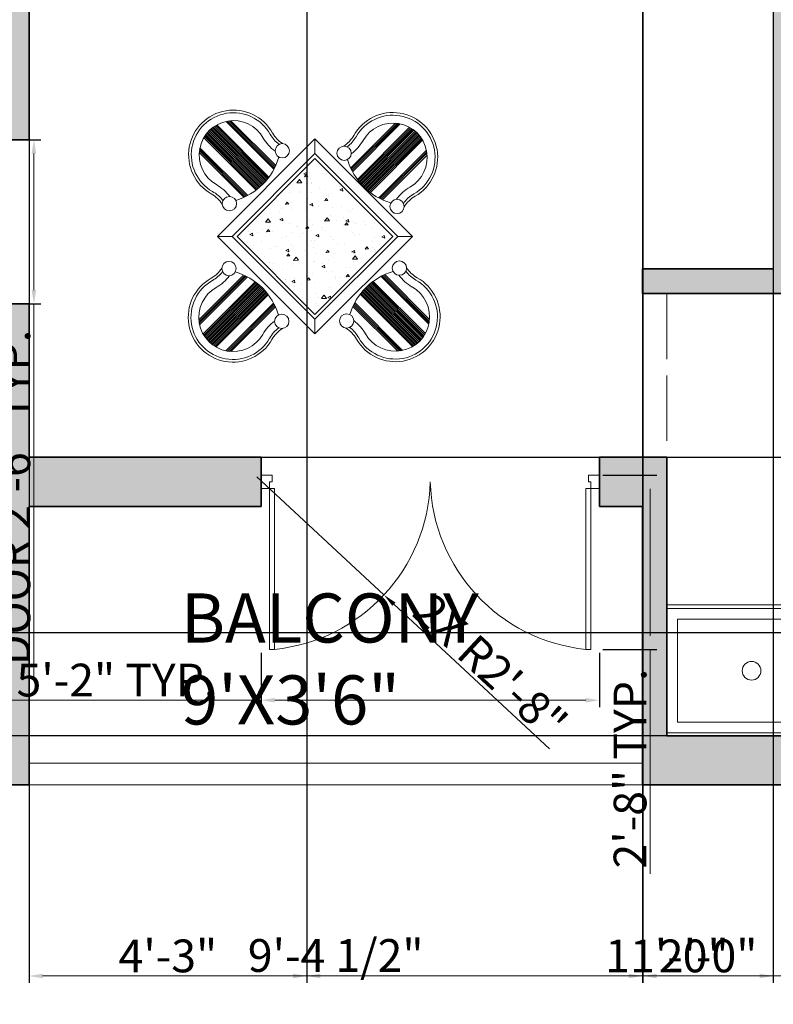
# Model space of a CAD drawing. Units: inches. Extents: x 2696 to 3240, y 1564 to 2310.
# Tile 25 of 76: x 2964 to 3102, y 1565 to 1745. Entities that reach past the tile are written whole.
import ezdxf

# ---------------------------------------------------------------- set-up
doc = ezdxf.new("R2010")
doc.units = ezdxf.units.IN
doc.linetypes.add('ACAD_ISO02W100', pattern=[15, 12, -3])
for name, color, linetype, lineweight in [('A-ANNO-DIMS', 3, 'Continuous', 18), ('A-AREA-IDEN', 7, 'Continuous', 18), ('A-DOOR', 4, 'Continuous', 18), ('A-FLOR-CASE', 8, 'Continuous', 18), ('A-FLOR-FIXT', 8, 'Continuous', 18), ('A-FLOR-HRAL', 7, 'Continuous', 18), ('A-FURN', 251, 'Continuous', 13), ('A-WALL', 7, 'Continuous', 35), ('A-WALL-OVHD', 7, 'ACAD_ISO02W100', 18), ('A-WALL-PATT', 9, 'Continuous', 13)]:
    doc.layers.add(name, color=color, linetype=linetype, lineweight=lineweight)
doc.styles.add('TIMES NEW', font='times.ttf')
doc.styles.add('YQ_DIM', font='SUPEROS.SHX', dxfattribs={"width": 0.8, "bigfont": 'HZDX.SHX'})
doc.dimstyles.new('Siddhuu', dxfattribs={"dimtxt": 6, "dimasz": 2.5, "dimexe": 1.25, "dimexo": 0.625, "dimtad": 1, "dimdec": 1, "dimlunit": 4, "dimtxsty": 'TIMES NEW', "dimcen": 2.5, "dimclrd": 256, "dimclre": 1, "dimclrt": 7, "dimadec": 0, "dimazin": 0, "dimtfac": 1, "dimtdec": 1, "dimtmove": 0, "dimatfit": 3, "dimfxl": 1, "dimtolj": 1, "dimlwd": -1, "dimarcsym": 0})

# ---------------------------------------------------------------- blocks, each defined once
blk = doc.blocks.new('DR_D02')
for p, q in [((-0.46, 0.4948), (-0.475, 0.4948)), ((-0.475, 0.02), (-0.475, 0.4948)), ((-0.46, 0.02), (-0.46, 0.495)), ((0.46, 0.02), (0.46, 0.495)), ((0.46, 0.4948), (0.475, 0.4948)), ((0.475, 0.02), (0.475, 0.4948)), ((-0.46, 0.02), (-0.5, 0.02)), ((-0.5, 0.02), (-0.5, -0.02)), ((-0.475, 0.02), (-0.475, 0)), ((-0.475, 0), (-0.4675, 0)), ((-0.4675, 0), (-0.4675, -0.02)), ((0.46, 0.02), (0.5, 0.02)), ((0.4675, 0), (0.4675, -0.02)), ((0.475, 0), (0.4675, 0)), ((0.475, 0.02), (0.475, 0)), ((0.5, 0.02), (0.5, -0.02)), ((-0.4675, -0.02), (-0.5, -0.02)), ((0.4675, -0.02), (0.5, -0.02))]:
    blk.add_line(p, q)
for centre, start, end in [((-0.5121, -0.0149), 1.6619, 84.1677), ((0.5121, -0.0149), 95.8323, 178.3381)]:
    blk.add_arc(centre, 0.5123, start, end)
blk = doc.blocks.new('DINING-SET-4')
h = blk.add_hatch()
h.set_pattern_fill('AR-CONC,_O', color=256, scale=0.03156, angle=135)
h.set_pattern_definition([(185, (694.1166, -47.9622), (-3.709933, 4.421326), [0.60121, -6.613307]), (130, (694.1166, -47.962), (-3.47714, -5.050095), [0.48097, -5.290645]), (235.451, (693.8074, -47.594), (-7.187067, -0.628735), [0.51095, -5.620443]), (181.1842, (692.983, -49.096), (-5.11118, 6.98761), [0.90181, -9.91996]), (231.6356, (692.557, -48.514), (-10.81945, -0.22364), [0.76642, -8.43066]), (126.184, (692.983, -49.096), (-10.81945, -0.22362), [0.72145, -7.93597]), (156, (692.6995, -48.2457), (-1.10128, 5.66559), [0.60121, -6.613307]), (101, (692.6995, -48.2457), (-5.48951, -2.73116), [0.48097, -5.290645]), (206.4514, (692.608, -47.7735), (-6.590787, 2.93441), [0.51095, -5.620443]), (172.5, (694.1166, -47.9622), (-1.955854, -1.8180035), [0, -5.226516, 0, -5.370807, 0, -5.310686]), (142.5, (694.1166, -47.9622), (-3.726774, -0.744482), [0, -3.062161, 0, -5.106274, 0, -2.024073]), (102.5, (695.3806, -49.2263), (-2.8979947, 3.15368), [0, -2.004032, 0, -6.25258, 0, -8.296694]), (92.5, (695.9475, -49.793), (-3.873065, 2.73823), [0, -2.605242, 0, -4.152355, 0, -5.891855])])
h.paths.add_polyline_path([(23.22, 8.74), (37.5, 23.02), (23.22, 37.31), (8.94, 23.02)])
for p, q in [((14.65, 33.71), (5.03, 43.33)), ((14.79, 33.91), (5.25, 43.45)), ((15.69, 35.33), (6.93, 44.09)), ((15.81, 35.56), (7.22, 44.15)), ((15.92, 35.79), (7.52, 44.19)), ((16.03, 36.02), (7.83, 44.22)), ((29.77, 35.57), (37.97, 43.77)), ((29.88, 35.34), (38.28, 43.74)), ((29.99, 35.11), (38.58, 43.7)), ((30.11, 34.88), (38.86, 43.64)), ((12.8, 31.8), (3.1, 41.5)), ((12.99, 31.96), (3.24, 41.7)), ((13.17, 32.12), (3.39, 41.89)), ((13.35, 32.28), (3.55, 42.08)), ((13.52, 32.45), (3.71, 42.26)), ((13.69, 32.62), (3.88, 42.43)), ((13.86, 32.79), (4.05, 42.6)), ((14.03, 32.97), (4.24, 42.76)), ((14.19, 33.15), (4.42, 42.91)), ((14.34, 33.33), (4.62, 43.06)), ((14.5, 33.52), (4.82, 43.2)), ((31, 33.46), (40.55, 43.01)), ((31.15, 33.26), (40.76, 42.88)), ((31.3, 33.07), (40.97, 42.75)), ((31.45, 32.88), (41.18, 42.61)), ((31.61, 32.7), (41.37, 42.46)), ((31.77, 32.52), (41.56, 42.31)), ((31.93, 32.34), (41.74, 42.15)), ((32.1, 32.17), (41.92, 41.98)), ((32.27, 32), (42.09, 41.81)), ((32.45, 31.83), (42.25, 41.63)), ((12.42, 31.5), (2.84, 41.08)), ((12.61, 31.65), (2.97, 41.3)), ((23.22, 38.2), (23.22, 40.88)), ((32.63, 31.67), (42.4, 41.45)), ((32.81, 31.51), (42.55, 41.25)), ((32.99, 31.35), (42.69, 41.05)), ((33.18, 31.2), (42.83, 40.85)), ((33.38, 31.05), (42.96, 40.63)), ((10.21, 30.19), (2.02, 38.38)), ((10.44, 30.3), (2.05, 38.7)), ((10.67, 30.41), (2.09, 39)), ((10.9, 30.53), (2.15, 39.28)), ((34.9, 30.08), (43.65, 38.83)), ((35.12, 29.96), (43.7, 38.55)), ((35.35, 29.85), (43.75, 38.25)), ((35.58, 29.74), (43.78, 37.94)), ((8.05, 23.02), (5.37, 23.02)), ((38.4, 23.02), (41.07, 23.02)), ((10.15, 15.95), (1.95, 7.75)), ((10.38, 15.84), (1.98, 7.44)), ((10.61, 15.73), (2.02, 7.14)), ((10.84, 15.61), (2.08, 6.86)), ((12.26, 14.72), (2.71, 5.17)), ((12.46, 14.57), (2.84, 4.95)), ((33.51, 14.5), (43.19, 4.83)), ((33.7, 14.65), (43.32, 5.04)), ((33.9, 14.8), (43.45, 5.25)), ((35.33, 15.7), (44.08, 6.94)), ((35.55, 15.81), (44.14, 7.23)), ((35.78, 15.93), (44.18, 7.52)), ((36.01, 16.03), (44.21, 7.83)), ((12.65, 14.42), (2.97, 4.75)), ((12.83, 14.27), (3.11, 4.54)), ((13.02, 14.11), (3.26, 4.35)), ((13.2, 13.95), (3.41, 4.16)), ((13.38, 13.78), (3.57, 3.98)), ((13.55, 13.62), (3.74, 3.8)), ((13.72, 13.45), (3.91, 3.63)), ((13.89, 13.27), (4.09, 3.47)), ((14.05, 13.09), (4.27, 3.32)), ((14.21, 12.91), (4.47, 3.17)), ((14.36, 12.72), (4.67, 3.03)), ((31.8, 12.81), (41.5, 3.11)), ((31.95, 12.99), (41.69, 3.25)), ((32.11, 13.18), (41.89, 3.4)), ((32.27, 13.35), (42.07, 3.55)), ((32.44, 13.53), (42.25, 3.72)), ((32.61, 13.7), (42.42, 3.89)), ((32.78, 13.87), (42.59, 4.06)), ((32.96, 14.03), (42.75, 4.24)), ((33.14, 14.19), (42.9, 4.43)), ((33.33, 14.35), (43.05, 4.63)), ((14.52, 12.54), (4.87, 2.89)), ((14.67, 12.34), (5.08, 2.76)), ((15.64, 10.82), (6.89, 2.07)), ((30.52, 10.91), (39.27, 2.15)), ((31.49, 12.43), (41.08, 2.85)), ((31.64, 12.62), (41.29, 2.97)), ((15.75, 10.6), (7.17, 2.02)), ((15.87, 10.37), (7.47, 1.97)), ((15.98, 10.14), (7.78, 1.94)), ((30.18, 10.22), (38.38, 2.03)), ((30.29, 10.45), (38.69, 2.06)), ((30.41, 10.68), (38.99, 2.1)), ((23.22, 7.85), (23.22, 5.17))]:
    blk.add_line(p, q)
for points in [[(41.07, 23.02), (23.22, 40.88), (5.37, 23.02), (23.22, 5.17)], [(38.4, 23.02), (23.22, 38.2), (8.05, 23.02), (23.22, 7.85)], [(37.5, 23.02), (23.22, 37.31), (8.94, 23.02), (23.22, 8.74)]]:
    blk.add_lwpolyline(points, close=True)
for centre in [(17.23, 38.71), (28.57, 38.26), (7.55, 29.03), (38.27, 28.51), (7.46, 17.15), (38.7, 17.23), (17.14, 7.47), (29.03, 7.55)]:
    blk.add_circle(centre, 1.31)
for centre, radius, start, end in [((8.28, 37.96), 8.21, 29.1881, 240.1532), ((8.28, 37.96), 7.72, 29.1881, 240.1532), ((37.51, 37.51), 8.21, 299.8468, 150.8119), ((37.51, 37.51), 7.72, 299.8468, 150.8119), ((8.28, 37.96), 6.28, 29.2752, 240.1505), ((37.51, 37.51), 6.28, 299.8495, 150.7248), ((20.45, 44.88), 6.28, 210.1015, 232.6572), ((20.45, 44.88), 5.79, 210.1015, 236.9513), ((25.34, 44.43), 5.79, 303.0487, 329.8985), ((20.45, 44.88), 7.72, 209.8594, 234.0675), ((25.34, 44.43), 6.28, 307.3428, 329.8985), ((25.34, 44.43), 7.72, 305.9325, 330.1406), ((5.4, 40.81), 11.66, 286.5158, 343.8317), ((40.4, 40.36), 11.66, 196.1683, 253.4842), ((1.37, 25.79), 7.72, 36.1055, 60.6071), ((1.37, 25.79), 5.79, 32.6748, 60.7093), ((1.37, 25.79), 6.28, 37.2611, 60.7093), ((44.43, 25.34), 7.72, 119.3929, 143.8945), ((44.43, 25.34), 6.28, 119.2907, 142.7389), ((44.43, 25.34), 5.79, 119.2907, 147.3252), ((1.29, 20.38), 5.79, 300.1015, 326.9513), ((1.29, 20.38), 6.28, 300.1015, 322.6572), ((5.36, 5.32), 11.66, 16.5158, 73.8317), ((40.8, 5.4), 11.66, 106.1683, 163.4842), ((44.87, 20.46), 6.28, 217.3428, 239.8985), ((44.87, 20.46), 5.79, 213.0487, 239.8985), ((8.21, 8.21), 8.21, 119.1881, 330.1532), ((8.21, 8.21), 7.72, 119.1881, 330.1532), ((1.29, 20.38), 7.72, 299.8594, 324.0675), ((37.95, 8.29), 8.21, 209.8468, 60.8119), ((37.95, 8.29), 7.72, 209.8468, 60.8119), ((44.87, 20.46), 7.72, 215.9325, 240.1406), ((8.21, 8.21), 6.28, 119.2752, 330.1505), ((37.95, 8.29), 6.28, 209.8495, 60.7248), ((20.38, 1.29), 7.72, 126.1055, 150.6071), ((25.78, 1.37), 7.72, 29.3929, 53.8945), ((20.38, 1.29), 6.28, 127.2611, 150.7093), ((20.38, 1.29), 5.79, 122.6748, 150.7093), ((25.78, 1.37), 5.79, 29.2907, 57.3252), ((25.78, 1.37), 6.28, 29.2907, 52.7389)]:
    blk.add_arc(centre, radius, start, end)
blk = doc.blocks.new('SINK-KITCHEN')
for points in [[(0, 22.8), (31.04, 22.8), (31.04, 0), (0, 0)], [(1.97, 20.82), (29.07, 20.82), (29.07, 1.97), (1.97, 1.97)]]:
    blk.add_lwpolyline(points, close=True)
blk.add_circle((15.52, 11.4), 1.71)
blk = doc.blocks.new('*D32')
at = {"layer": 'A-ANNO-DIMS', "color": 1, "lineweight": -2, "transparency": 16777216}
for p, q in [((2962.73, 1723.33), (2967.86, 1723.33)), ((2962.73, 1693.33), (2967.86, 1693.33))]:
    blk.add_line(p, q, dxfattribs=at)
at = {"layer": 'A-ANNO-DIMS', "transparency": 16777216}
for p, q in [((2966.61, 1720.83), (2966.61, 1695.83)), ((2966.61, 1693.33), (2966.61, 1624.85))]:
    blk.add_line(p, q, dxfattribs=at)
for points in [[(2966.19, 1720.83), (2967.03, 1720.83), (2966.61, 1723.33)], [(2966.19, 1695.83), (2967.03, 1695.83), (2966.61, 1693.33)]]:
    blk.add_solid(points, dxfattribs=at)
at = {"layer": 'Defpoints', "color": 0, "transparency": 16777216}
for p in [(2962.11, 1723.33), (2962.11, 1693.33), (2966.61, 1693.33)]:
    blk.add_point(p, dxfattribs=at)
at = {"layer": 'A-ANNO-DIMS', "color": 7, "transparency": 16777216, "insert": (2962.92, 1657.84), "char_height": 6, "attachment_point": 5, "rotation": 90, "style": 'TIMES NEW'}
blk.add_mtext('\\A1;DOOR 2\'-6" TYP.', dxfattribs=at)
blk = doc.blocks.new('*D36')
at = {"layer": 'A-ANNO-DIMS', "color": 1, "lineweight": -2, "transparency": 16777216}
for p, q in [((3008.24, 1629.39), (3008.24, 1619.46)), ((3070.24, 1629.39), (3070.24, 1619.46))]:
    blk.add_line(p, q, dxfattribs=at)
at = {"layer": 'A-ANNO-DIMS', "transparency": 16777216}
for p, q in [((3008.24, 1620.71), (2894.72, 1620.71)), ((3067.74, 1620.71), (3010.74, 1620.71))]:
    blk.add_line(p, q, dxfattribs=at)
for points in [[(3010.74, 1621.13), (3010.74, 1620.29), (3008.24, 1620.71)], [(3067.74, 1621.13), (3067.74, 1620.29), (3070.24, 1620.71)]]:
    blk.add_solid(points, dxfattribs=at)
at = {"layer": 'Defpoints', "color": 0, "transparency": 16777216}
for p in [(3008.24, 1630.01), (3070.24, 1630.01), (3008.24, 1620.71)]:
    blk.add_point(p, dxfattribs=at)
at = {"layer": 'A-ANNO-DIMS', "color": 7, "transparency": 16777216, "insert": (2950.23, 1624.4), "char_height": 6, "attachment_point": 5, "style": 'TIMES NEW'}
blk.add_mtext('\\A1;BALCONY DOOR 5\'-2" TYP.', dxfattribs=at)
blk = doc.blocks.new('*D37')
at = {"layer": 'A-ANNO-DIMS', "color": 1, "lineweight": -2, "transparency": 16777216}
for p, q in [((3070.86, 1661.94), (3080.79, 1661.94)), ((3070.86, 1630.01), (3080.79, 1630.01))]:
    blk.add_line(p, q, dxfattribs=at)
at = {"layer": 'A-ANNO-DIMS', "transparency": 16777216}
for p, q in [((3079.54, 1659.44), (3079.54, 1632.51)), ((3079.54, 1630.01), (3079.54, 1588.89))]:
    blk.add_line(p, q, dxfattribs=at)
for points in [[(3079.12, 1659.44), (3079.95, 1659.44), (3079.54, 1661.94)], [(3079.12, 1632.51), (3079.95, 1632.51), (3079.54, 1630.01)]]:
    blk.add_solid(points, dxfattribs=at)
at = {"layer": 'Defpoints', "color": 0, "transparency": 16777216}
for p in [(3070.24, 1661.94), (3070.24, 1630.01), (3079.54, 1630.01)]:
    blk.add_point(p, dxfattribs=at)
at = {"layer": 'A-ANNO-DIMS', "color": 7, "transparency": 16777216, "insert": (3075.85, 1608.2), "char_height": 6, "attachment_point": 5, "rotation": 90, "style": 'TIMES NEW'}
blk.add_mtext('\\A1;2\'-8" TYP.', dxfattribs=at)
blk = doc.blocks.new('*D50')
at = {"layer": 'A-ANNO-DIMS', "color": 1, "lineweight": -2, "transparency": 16777216}
for p, q in [((2965.71, 1979.58), (2965.71, 1568.95)), ((3016.61, 1979.58), (3016.61, 1568.95))]:
    blk.add_line(p, q, dxfattribs=at)
at = {"layer": 'A-ANNO-DIMS', "transparency": 16777216}
blk.add_line((2968.21, 1570.2), (3014.11, 1570.2), dxfattribs=at)
for points in [[(2968.21, 1570.62), (2968.21, 1569.78), (2965.71, 1570.2)], [(3014.11, 1570.62), (3014.11, 1569.78), (3016.61, 1570.2)]]:
    blk.add_solid(points, dxfattribs=at)
at = {"layer": 'Defpoints', "color": 0, "transparency": 16777216}
for p in [(2965.71, 1980.2), (3016.61, 1980.2), (3016.61, 1570.2)]:
    blk.add_point(p, dxfattribs=at)
at = {"layer": 'A-ANNO-DIMS', "color": 7, "transparency": 16777216, "insert": (2991.16, 1573.88), "char_height": 6, "attachment_point": 5, "style": 'TIMES NEW'}
blk.add_mtext('\\A1;4\'-3"', dxfattribs=at)
blk = doc.blocks.new('*D51')
at = {"layer": 'A-ANNO-DIMS', "color": 1, "lineweight": -2, "transparency": 16777216}
for p, q in [((3016.61, 1979.58), (3016.61, 1568.95)), ((3148.61, 1979.58), (3148.61, 1568.95))]:
    blk.add_line(p, q, dxfattribs=at)
at = {"layer": 'A-ANNO-DIMS', "transparency": 16777216}
blk.add_line((3019.11, 1570.2), (3146.11, 1570.2), dxfattribs=at)
for points in [[(3019.11, 1570.62), (3019.11, 1569.78), (3016.61, 1570.2)], [(3146.11, 1570.62), (3146.11, 1569.78), (3148.61, 1570.2)]]:
    blk.add_solid(points, dxfattribs=at)
at = {"layer": 'Defpoints', "color": 0, "transparency": 16777216}
for p in [(3016.61, 1980.2), (3148.61, 1980.2), (3148.61, 1570.2)]:
    blk.add_point(p, dxfattribs=at)
at = {"layer": 'A-ANNO-DIMS', "color": 7, "transparency": 16777216, "insert": (3082.61, 1573.88), "char_height": 6, "attachment_point": 5, "style": 'TIMES NEW'}
blk.add_mtext('\\A1;11\'-0"', dxfattribs=at)
blk = doc.blocks.new('*D56')
at = {"layer": 'A-ANNO-DIMS', "color": 1, "lineweight": -2, "transparency": 16777216}
for p, q in [((2966.33, 1884.2), (3235.86, 1884.2)), ((2966.33, 1665.2), (3235.86, 1665.2))]:
    blk.add_line(p, q, dxfattribs=at)
at = {"layer": 'A-ANNO-DIMS', "transparency": 16777216}
blk.add_line((3234.61, 1667.7), (3234.61, 1881.7), dxfattribs=at)
for points in [[(3234.19, 1881.7), (3235.03, 1881.7), (3234.61, 1884.2)], [(3234.19, 1667.7), (3235.03, 1667.7), (3234.61, 1665.2)]]:
    blk.add_solid(points, dxfattribs=at)
at = {"layer": 'Defpoints', "color": 0, "transparency": 16777216}
for p in [(2965.71, 1884.2), (3234.61, 1884.2), (2965.71, 1665.2)]:
    blk.add_point(p, dxfattribs=at)
at = {"layer": 'A-ANNO-DIMS', "color": 7, "transparency": 16777216, "insert": (3230.93, 1774.7), "char_height": 6, "attachment_point": 5, "rotation": 90, "style": 'TIMES NEW'}
blk.add_mtext('\\A1;18\'-3"', dxfattribs=at)
blk = doc.blocks.new('*D65')
at = {"layer": 'A-ANNO-DIMS', "color": 1, "lineweight": -2, "transparency": 16777216}
for p, q in [((3078.21, 2122.08), (3078.21, 1568.95)), ((3102.11, 2122.08), (3102.11, 1568.95))]:
    blk.add_line(p, q, dxfattribs=at)
at = {"layer": 'A-ANNO-DIMS', "transparency": 16777216}
blk.add_line((3080.71, 1570.2), (3099.61, 1570.2), dxfattribs=at)
for points in [[(3080.71, 1570.62), (3080.71, 1569.78), (3078.21, 1570.2)], [(3099.61, 1570.62), (3099.61, 1569.78), (3102.11, 1570.2)]]:
    blk.add_solid(points, dxfattribs=at)
at = {"layer": 'Defpoints', "color": 0, "transparency": 16777216}
for p in [(3078.21, 2122.7), (3102.11, 2122.7), (3102.11, 1570.2)]:
    blk.add_point(p, dxfattribs=at)
at = {"layer": 'A-ANNO-DIMS', "color": 7, "transparency": 16777216, "insert": (3090.16, 1573.88), "char_height": 6, "attachment_point": 5, "style": 'TIMES NEW'}
blk.add_mtext('\\A1;2\'-0"', dxfattribs=at)
blk = doc.blocks.new('*D67')
at = {"layer": 'A-ANNO-DIMS', "color": 1, "lineweight": -2, "transparency": 16777216}
for p, q in [((2965.71, 1883.58), (2965.71, 1568.95)), ((3078.11, 1791.45), (3078.11, 1568.95))]:
    blk.add_line(p, q, dxfattribs=at)
at = {"layer": 'A-ANNO-DIMS', "transparency": 16777216}
blk.add_line((2968.21, 1570.2), (3075.61, 1570.2), dxfattribs=at)
for points in [[(2968.21, 1570.62), (2968.21, 1569.78), (2965.71, 1570.2)], [(3075.61, 1570.62), (3075.61, 1569.78), (3078.11, 1570.2)]]:
    blk.add_solid(points, dxfattribs=at)
at = {"layer": 'Defpoints', "color": 0, "transparency": 16777216}
for p in [(2965.71, 1884.2), (3078.11, 1792.08), (3078.11, 1570.2)]:
    blk.add_point(p, dxfattribs=at)
at = {"layer": 'A-ANNO-DIMS', "color": 7, "transparency": 16777216, "insert": (3021.91, 1573.96), "char_height": 6, "attachment_point": 5, "style": 'TIMES NEW'}
blk.add_mtext('\\A1;9\'-4 1/2"', dxfattribs=at)
blk = doc.blocks.new('*D81')
at = {"layer": 'A-ANNO-DIMS', "color": 1, "lineweight": -2, "transparency": 16777216}
for p, q in [((3189.99, 1633.05), (2709.36, 1633.05)), ((3189.99, 1614.2), (2709.36, 1614.2))]:
    blk.add_line(p, q, dxfattribs=at)
at = {"layer": 'A-ANNO-DIMS', "transparency": 16777216}
blk.add_line((2710.61, 1616.7), (2710.61, 1630.55), dxfattribs=at)
for points in [[(2710.19, 1630.55), (2711.03, 1630.55), (2710.61, 1633.05)], [(2710.19, 1616.7), (2711.03, 1616.7), (2710.61, 1614.2)]]:
    blk.add_solid(points, dxfattribs=at)
at = {"layer": 'Defpoints', "color": 0, "transparency": 16777216}
for p in [(2710.61, 1633.05), (3190.61, 1633.05), (3190.61, 1614.2)]:
    blk.add_point(p, dxfattribs=at)
at = {"layer": 'A-ANNO-DIMS', "color": 7, "transparency": 16777216, "insert": (2706.93, 1623.62), "char_height": 6, "attachment_point": 5, "rotation": 90, "style": 'TIMES NEW'}
blk.add_mtext('\\A1;1\'-7"', dxfattribs=at)
blk = doc.blocks.new('*D84')
at = {"layer": 'A-ANNO-DIMS', "transparency": 16777216}
for p, q in [((3007.49, 1661.62), (3030.75, 1640)), ((3061.1, 1611.78), (3032.58, 1638.29))]:
    blk.add_line(p, q, dxfattribs=at)
blk.add_solid([(3032.87, 1638.6), (3032.3, 1637.99), (3030.75, 1640)], dxfattribs=at)
at = {"layer": 'Defpoints', "color": 0, "transparency": 16777216}
for p in [(3007.49, 1661.62), (3030.75, 1640)]:
    blk.add_point(p, dxfattribs=at)
at = {"layer": 'A-ANNO-DIMS', "color": 7, "transparency": 16777216, "insert": (3050.26, 1626.88), "char_height": 6, "attachment_point": 5, "rotation": 317.0859, "style": 'TIMES NEW'}
blk.add_mtext('\\A1;2X R2\'-8"', dxfattribs=at)

msp = doc.modelspace()

# ---------------------------------------------------------------- hatches: boundary and pattern name
at = {"layer": 'A-WALL-PATT', "transparency": 33554556}
h = msp.add_hatch(color=256, dxfattribs=at)
h.dxf.hatch_style = 1
h.paths.add_polyline_path([(2879.11, 2253.2), (2905.91, 2253.2), (2905.91, 2262.2), (2841.89, 2262.2), (2841.89, 2253.2), (2870.11, 2253.2), (2870.11, 2176.6), (2965.71, 2176.6), (2965.71, 2206.7), (2973.58, 2206.7), (2973.58, 2215.7), (2965.71, 2215.7), (2965.71, 2262.2), (2929.91, 2262.2), (2929.91, 2253.2), (2956.71, 2253.2), (2956.71, 2185.6), (2879.11, 2185.6)])
h.paths.add_polyline_path([(2782.83, 2262.2), (2745.61, 2262.2), (2745.61, 2228.73), (2754.61, 2228.73), (2754.61, 2253.2), (2782.83, 2253.2)])
h.paths.add_polyline_path([(2754.61, 2136.2), (2965.71, 2136.2), (2965.71, 2145.2), (2879.11, 2145.2), (2879.11, 2147.07), (2877.34, 2147.07), (2870.11, 2147.07), (2870.11, 2145.2), (2754.61, 2145.2), (2754.61, 2169.67), (2745.61, 2169.67), (2745.61, 2000.2), (2754.61, 2000.2), (2754.61, 2019.2), (2849.08, 2019.2), (2849.08, 2023.7), (2841.21, 2023.7), (2841.21, 2051.83), (2836.71, 2051.83), (2836.71, 2023.7), (2754.61, 2023.7), (2754.61, 2091.2), (2836.71, 2091.2), (2836.71, 2087.83), (2841.21, 2087.83), (2841.21, 2095.7), (2754.61, 2095.7)])
h.paths.add_polyline_path([(2965.71, 2136.2), (2956.71, 2136.2), (2956.71, 2023.7), (2885.08, 2023.7), (2885.08, 2019.2), (2956.71, 2019.2), (2956.71, 1950.58), (2965.71, 1950.58), (2965.71, 1980.2), (2973.58, 1980.2), (2973.58, 1989.2), (2965.71, 1989.2)])
h.paths.add_polyline_path([(2754.61, 1906.7), (2880.21, 1906.7), (2884.71, 1906.7), (2956.71, 1906.7), (2956.71, 1792.7), (2944.71, 1792.7), (2944.71, 1783.7), (2956.71, 1783.7), (2956.71, 1740.2), (2884.71, 1740.2), (2884.71, 1783.7), (2896.71, 1783.7), (2896.71, 1792.7), (2884.71, 1792.7), (2884.71, 1846.7), (2880.21, 1846.7), (2880.21, 1740.2), (2754.61, 1740.2), (2754.61, 1777.2), (2745.61, 1777.2), (2745.61, 1692.7), (2754.61, 1692.7), (2754.61, 1731.2), (2956.71, 1731.2), (2956.71, 1723.33), (2965.71, 1723.33), (2965.71, 1884.2), (2973.58, 1884.2), (2973.58, 1893.2), (2965.71, 1893.2), (2965.71, 1914.58), (2956.71, 1914.58), (2956.71, 1911.2), (2754.61, 1911.2), (2754.61, 1930.2), (2745.61, 1930.2), (2745.61, 1817.2), (2754.61, 1817.2), (2754.61, 1854.2), (2826.61, 1854.2), (2826.61, 1868.83), (2822.11, 1868.83), (2822.11, 1858.7), (2754.61, 1858.7)])
h.paths.add_polyline_path([(2965.71, 1656.2), (3008.24, 1656.2), (3008.24, 1665.2), (2965.71, 1665.2), (2965.71, 1693.33), (2956.71, 1693.33), (2956.71, 1686.2), (2934.58, 1686.2), (2934.58, 1681.7), (2956.71, 1681.7), (2956.71, 1614.2), (2896.71, 1614.2), (2896.71, 1681.7), (2904.58, 1681.7), (2904.58, 1686.2), (2892.21, 1686.2), (2892.21, 1614.2), (2858.41, 1614.2), (2858.41, 1605.2), (2965.71, 1605.2)])
h.paths.add_polyline_path([(2788.41, 1614.2), (2754.61, 1614.2), (2754.61, 1652.7), (2745.61, 1652.7), (2745.61, 1605.2), (2788.41, 1605.2)])
h.paths.add_polyline_path([(3199.61, 1633.05), (3190.61, 1633.05), (3190.61, 1614.2), (3082.61, 1614.2), (3082.61, 1665.2), (3070.24, 1665.2), (3070.24, 1656.2), (3078.11, 1656.2), (3078.11, 1605.2), (3199.61, 1605.2)])
h.paths.add_polyline_path([(3199.61, 1702.05), (3190.61, 1702.05), (3190.61, 1699.7), (3106.61, 1699.7), (3106.61, 1747.7), (3190.61, 1747.7), (3190.61, 1752.2), (3082.61, 1752.2), (3082.61, 1760.08), (3078.11, 1760.08), (3078.11, 1747.7), (3102.11, 1747.7), (3102.11, 1699.7), (3078.11, 1699.7), (3078.11, 1695.2), (3190.61, 1695.2), (3190.61, 1676.35), (3199.61, 1676.35)])
h.paths.add_polyline_path([(3199.61, 1783.2), (3190.61, 1783.2), (3190.61, 1745.35), (3199.61, 1745.35)])
h.paths.add_polyline_path([(3082.61, 1884.2), (3190.61, 1884.2), (3190.61, 1853.2), (3199.61, 1853.2), (3199.61, 1901.7), (3190.61, 1901.7), (3190.61, 1893.2), (3005.58, 1893.2), (3005.58, 1891.28), (3005.58, 1884.2), (3078.11, 1884.2), (3078.11, 1792.08), (3082.61, 1792.08)])
h.paths.add_polyline_path([(3199.61, 1994.7), (3190.61, 1994.7), (3190.61, 1989.2), (3073.71, 1989.2), (3073.71, 2034.2), (3069.21, 2034.2), (3069.21, 1989.2), (3005.58, 1989.2), (3005.58, 1980.2), (3190.61, 1980.2), (3190.61, 1971.7), (3199.61, 1971.7)])
h.paths.add_polyline_path([(3199.61, 2155.2), (3190.61, 2155.2), (3190.61, 2064.7), (3199.61, 2064.7)])
h.paths.add_polyline_path([(3190.61, 2074.7), (3106.61, 2074.7), (3106.61, 2122.7), (3190.61, 2122.7), (3190.61, 2127.2), (3082.71, 2127.2), (3082.71, 2135.08), (3073.71, 2135.08), (3073.71, 2122.7), (3102.11, 2122.7), (3102.11, 2074.7), (3069.21, 2074.7), (3069.21, 2070.2), (3190.61, 2070.2)])
h.paths.add_polyline_path([(3082.71, 2253.2), (3190.61, 2253.2), (3190.61, 2225.2), (3199.61, 2225.2), (3199.61, 2262.2), (3073.71, 2262.2), (3073.71, 2215.7), (3035.58, 2215.7), (3035.58, 2206.7), (3073.71, 2206.7), (3073.71, 2171.08), (3082.71, 2171.08)])

# ---------------------------------------------------------------- linework, layer by layer
at = {"layer": 'A-FLOR-CASE'}
msp.add_line((3082.61, 1638.2), (3166.61, 1638.2), dxfattribs=at)
at = {"layer": 'A-FLOR-HRAL'}
for p, q in [((2965.71, 1609.2), (3078.11, 1609.2)), ((2965.71, 1605.2), (3078.11, 1605.2))]:
    msp.add_line(p, q, dxfattribs=at)
at = {"layer": 'A-WALL'}
for p, q in [((2965.71, 1884.2), (2965.71, 1723.33)), ((2956.71, 1723.33), (2965.71, 1723.33)), ((3078.11, 1699.7), (3102.11, 1699.7)), ((3078.11, 1695.2), (3078.11, 1699.7)), ((3078.11, 1695.2), (3190.61, 1695.2)), ((2956.71, 1693.33), (2965.71, 1693.33)), ((2965.71, 1693.33), (2965.71, 1665.2)), ((2965.71, 1665.2), (3008.24, 1665.2)), ((3008.24, 1665.2), (3008.24, 1656.2)), ((3070.24, 1665.2), (3082.61, 1665.2)), ((3070.24, 1665.2), (3070.24, 1656.2)), ((3082.61, 1614.2), (3082.61, 1665.2)), ((2965.71, 1656.2), (3008.24, 1656.2)), ((2965.71, 1656.2), (2965.71, 1605.2)), ((3070.24, 1656.2), (3078.11, 1656.2)), ((3078.11, 1605.2), (3078.11, 1656.2)), ((3082.61, 1614.2), (3190.61, 1614.2)), ((2858.41, 1605.2), (2965.71, 1605.2)), ((3078.11, 1605.2), (3199.61, 1605.2))]:
    msp.add_line(p, q, dxfattribs=at)
at = {"layer": 'A-WALL-OVHD'}
for p, q in [((3078.11, 1695.2), (3078.11, 1665.2)), ((3082.61, 1695.2), (3082.61, 1665.2))]:
    msp.add_line(p, q, dxfattribs=at)

# ---------------------------------------------------------------- block references
at = {"layer": 'A-DOOR', "xscale": 62, "yscale": 62, "zscale": 62, "rotation": 180.0000000000002}
msp.add_blockref('DR_D02', (3039.24, 1660.7), dxfattribs=at)
at = {"layer": 'A-FLOR-FIXT'}
msp.add_blockref('SINK-KITCHEN', (3082.61, 1614.71), dxfattribs=at)
at = {"layer": 'A-FURN'}
msp.add_blockref('DINING-SET-4', (2994.89, 1682.63), dxfattribs=at)

# ---------------------------------------------------------------- texts
at = {"layer": 'A-AREA-IDEN', "insert": (2993.57, 1640.27), "char_height": 9, "attachment_point": 1, "style": 'YQ_DIM'}
msp.add_mtext_dynamic_manual_height_columns('BALCONY\\P9\'X3\'6"', width=48.0032, gutter_width=12.5, heights=[0], dxfattribs=at)

# ---------------------------------------------------------------- dimensions: what is measured, and where the dimension line sits
at = {"layer": 'A-ANNO-DIMS'}
for base, p1, p2, picture, middle in [((3102.11, 1570.2), (3078.21, 2122.7), (3102.11, 2122.7), '*D65', (3090.16, 1573.88)), ((3016.61, 1570.2), (2965.71, 1980.2), (3016.61, 1980.2), '*D50', (2991.16, 1573.88)), ((3148.61, 1570.2), (3016.61, 1980.2), (3148.61, 1980.2), '*D51', (3082.61, 1573.88)), ((3078.11, 1570.2), (2965.71, 1884.2), (3078.11, 1792.08), '*D67', (3021.91, 1573.96))]:
    dim = msp.add_linear_dim(base=base, p1=p1, p2=p2, dimstyle='Siddhuu', override={"dimdec": 1, "dimlfac": 1, "dimrnd": 0, "dimzin": 1, "dimdsep": 46, "dimlunit": 4, "dimfrac": 2}, dxfattribs=at)
    dim.commit()
    dim.dimension.update_dxf_attribs({"geometry": picture, "text_midpoint": middle})
for base, p1, p2, picture, middle in [((3234.61, 1884.2), (2965.71, 1665.2), (2965.71, 1884.2), '*D56', (3230.93, 1774.7)), ((2710.6114, 1633.0476), (3190.6114, 1614.2011), (3190.6114, 1633.0476), '*D81', (2706.9258, 1623.6243))]:
    dim = msp.add_linear_dim(base=base, p1=p1, p2=p2, angle=90, dimstyle='Siddhuu', override={"dimdec": 1, "dimlfac": 1, "dimrnd": 0, "dimzin": 1, "dimdsep": 46, "dimlunit": 4, "dimfrac": 2}, dxfattribs=at)
    dim.commit()
    dim.dimension.update_dxf_attribs({"geometry": picture, "text_midpoint": middle})
for base, p1, p2, angle, text, picture, middle in [((2966.61, 1693.33), (2962.11, 1723.33), (2962.11, 1693.33), 270, 'DOOR <> TYP.', '*D32', (2962.92, 1657.84)), ((3079.54, 1630.01), (3070.24, 1661.94), (3070.24, 1630.01), 270, '<> TYP.', '*D37', (3075.85, 1608.2)), ((3008.24, 1620.71), (3070.24, 1630.01), (3008.24, 1630.01), 180, 'BALCONY DOOR <> TYP.', '*D36', (2950.23, 1624.4))]:
    dim = msp.add_linear_dim(base=base, p1=p1, p2=p2, angle=angle, text=text, dimstyle='Siddhuu', override={"dimdec": 1, "dimlfac": 1, "dimrnd": 0, "dimzin": 1, "dimdsep": 46, "dimlunit": 4, "dimfrac": 2}, dxfattribs=at)
    dim.commit()
    dim.dimension.update_dxf_attribs({"geometry": picture, "text_midpoint": middle})
dim = msp.add_radius_dim(center=(3007.49, 1661.62), mpoint=(3030.75, 1640), text='2X <>', dimstyle='Siddhuu', override={"dimdec": 1, "dimlfac": 1, "dimrnd": 0, "dimzin": 1, "dimdsep": 46, "dimlunit": 4, "dimfrac": 2}, dxfattribs=at)
dim.commit()
dim.dimension.update_dxf_attribs({"geometry": '*D84', "text_midpoint": (3050.26, 1626.88)})

doc.saveas('drawing.dxf')
